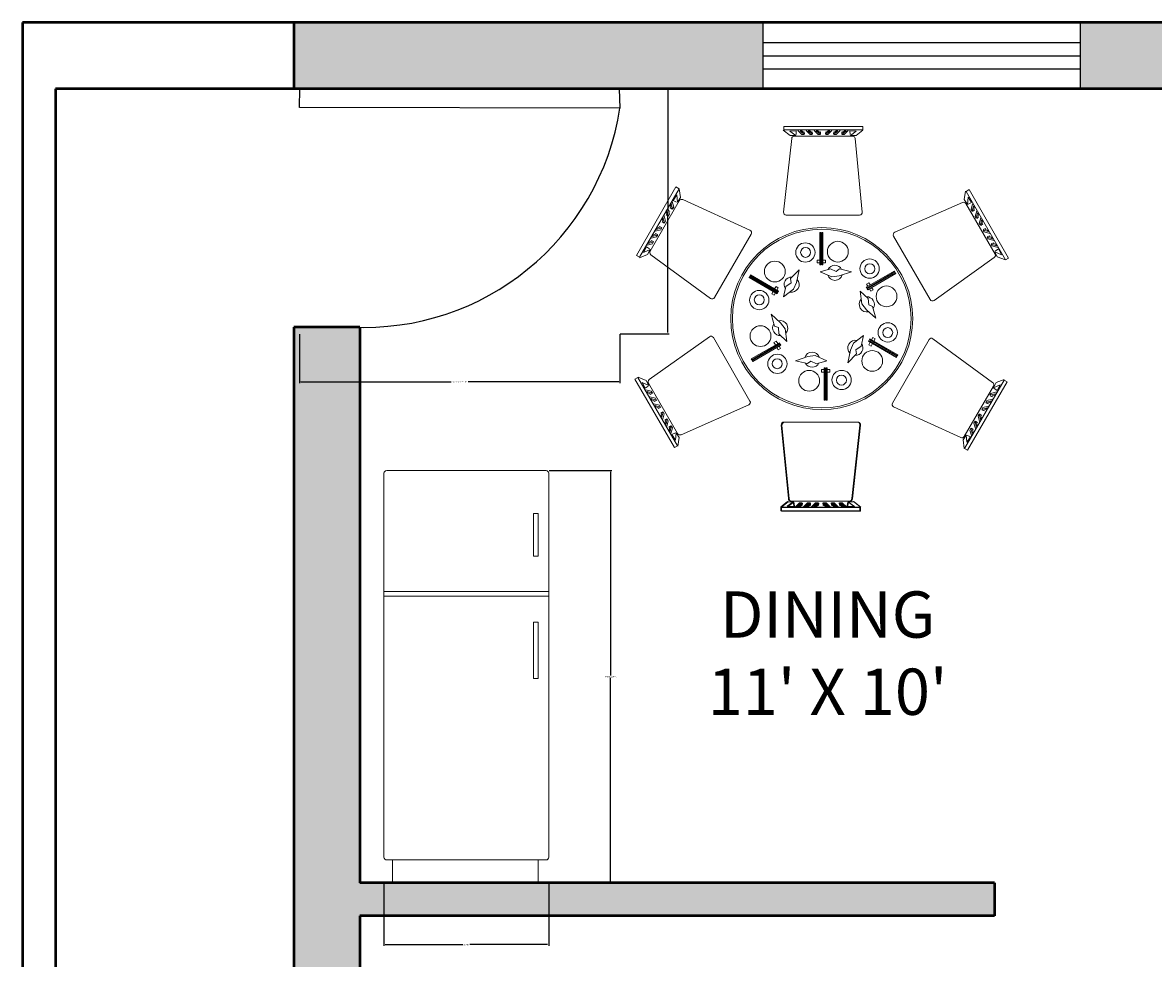
# Model space of a CAD drawing. Units: inches. Extents: x 1771 to 3025, y 319 to 889.
# Tile 19 of 35: x 2219 to 2390, y 747 to 889. Entities that reach past the tile are written whole.
import ezdxf

# ---------------------------------------------------------------- set-up
doc = ezdxf.new("R2010")
doc.units = ezdxf.units.IN
doc.header["$MEASUREMENT"] = 0
for name, color, linetype, lineweight in [('A-ANNO-DIMS', 2, 'Continuous', 18), ('A-AREA-IDEN', 241, 'Continuous', 25), ('A-DOOR', 4, 'Continuous', 25), ('A-FURN', 8, 'Continuous', 18), ('A-GLAZ', 40, 'Continuous', 25), ('A-WALL', 7, 'Continuous', 50), ('A-WALL-PATT', 254, 'Continuous', 13)]:
    doc.layers.add(name, color=color, linetype=linetype, lineweight=lineweight)
doc.styles.get("Standard").update_dxf_attribs({"font": 'arial.ttf'})
doc.dimstyles.get("Standard").update_dxf_attribs({"dimtxt": 0.18, "dimasz": 0.18, "dimexe": 0.18, "dimexo": 0.0625, "dimgap": 0.09, "dimtad": 0, "dimtih": 1, "dimtoh": 1, "dimdec": 4, "dimzin": 0, "dimdsep": 46, "dimtxsty": 'Standard', "dimcen": 0.09, "dimadec": 0, "dimazin": 0, "dimtfac": 1, "dimtdec": 4, "dimtofl": 0, "dimtmove": 0, "dimatfit": 3, "dimfxl": 1, "dimtolj": 1, "dimtzin": 0, "dimarcsym": 0})

# ---------------------------------------------------------------- blocks, each defined once
blk = doc.blocks.new('A$C1C317F9A')
for p, q in [((0.8756, 2.2462), (0.9155, 2.2143)), ((0.8788, 2.2685), (0.8788, 2.2478)), ((1.3449, 2.2685), (0.8788, 2.2685)), ((0.8788, 2.2478), (1.3449, 2.2478)), ((0.9139, 2.2414), (0.9522, 2.243)), ((0.949, 2.2159), (0.9139, 2.2414)), ((0.9155, 2.2143), (0.949, 2.2159)), ((0.941, 2.2111), (1.2841, 2.2111)), ((0.9522, 2.243), (0.9506, 2.2206)), ((0.9618, 2.2446), (0.9857, 2.2206)), ((0.9745, 2.243), (0.9841, 2.243)), ((0.9985, 2.2206), (0.9745, 2.243)), ((0.9841, 2.243), (0.9953, 2.2334)), ((0.9857, 2.2206), (0.9985, 2.2206)), ((0.9953, 2.2334), (0.9985, 2.2366)), ((0.9985, 2.2366), (1.0001, 2.2222)), ((1.0097, 2.2446), (1.0336, 2.2206)), ((1.0224, 2.243), (1.032, 2.243)), ((1.0464, 2.2206), (1.0224, 2.243)), ((1.032, 2.243), (1.0432, 2.2334)), ((1.0336, 2.2206), (1.0464, 2.2206)), ((1.0432, 2.2334), (1.0464, 2.2366)), ((1.0464, 2.2366), (1.048, 2.2222)), ((1.0576, 2.2446), (1.0815, 2.2206)), ((1.0703, 2.243), (1.0799, 2.243)), ((1.0943, 2.2206), (1.0703, 2.243)), ((1.0799, 2.243), (1.0911, 2.2334)), ((1.0815, 2.2206), (1.0943, 2.2206)), ((1.0911, 2.2334), (1.0943, 2.2366)), ((1.0943, 2.2366), (1.0959, 2.2222)), ((1.1262, 2.2366), (1.1246, 2.2222)), ((1.1262, 2.2206), (1.1502, 2.243)), ((1.1294, 2.2334), (1.1262, 2.2366)), ((1.139, 2.2206), (1.1262, 2.2206)), ((1.1406, 2.243), (1.1294, 2.2334)), ((1.1629, 2.2446), (1.139, 2.2206)), ((1.1502, 2.243), (1.1406, 2.243)), ((1.1741, 2.2366), (1.1725, 2.2222)), ((1.1741, 2.2206), (1.1981, 2.243)), ((1.1773, 2.2334), (1.1741, 2.2366)), ((1.1869, 2.2206), (1.1741, 2.2206)), ((1.1885, 2.243), (1.1773, 2.2334)), ((1.2108, 2.2446), (1.1869, 2.2206)), ((1.1981, 2.243), (1.1885, 2.243)), ((1.222, 2.2366), (1.2204, 2.2222)), ((1.222, 2.2206), (1.246, 2.243)), ((1.2252, 2.2334), (1.222, 2.2366)), ((1.2348, 2.2206), (1.222, 2.2206)), ((1.2364, 2.243), (1.2252, 2.2334)), ((1.2587, 2.2446), (1.2348, 2.2206)), ((1.246, 2.243), (1.2364, 2.243)), ((1.2683, 2.243), (1.2699, 2.2206)), ((1.3066, 2.2414), (1.2683, 2.243)), ((1.2715, 2.2159), (1.3066, 2.2414)), ((1.305, 2.2143), (1.2715, 2.2159)), ((1.3449, 2.2462), (1.305, 2.2143)), ((1.3449, 2.2478), (1.3449, 2.2685)), ((0.8775, 1.7628), (0.9251, 2.1968)), ((1.3, 2.1966), (1.3417, 1.7626)), ((0.2422, 1.9115), (0.0091, 1.5078)), ((0.0271, 1.4974), (0.2602, 1.9011)), ((0.2602, 1.9011), (0.2422, 1.9115)), ((0.2615, 1.9003), (0.2692, 1.8498)), ((1.9514, 1.8873), (1.9438, 1.8368)), ((1.9724, 1.8957), (1.9544, 1.8854)), ((1.9544, 1.8854), (2.1875, 1.4816)), ((2.2055, 1.492), (1.9724, 1.8957)), ((0.09, 1.5329), (0.2615, 1.8301)), ((0.2148, 1.813), (0.21, 1.8047)), ((0.21, 1.8047), (0.2127, 1.7903)), ((0.2222, 1.7811), (0.2148, 1.813)), ((0.2198, 1.8249), (0.2286, 1.7922)), ((0.2465, 1.8648), (0.226, 1.8324)), ((0.226, 1.8324), (0.2461, 1.8226)), ((0.2511, 1.8216), (0.2465, 1.8648)), ((0.2692, 1.8498), (0.2511, 1.8216)), ((0.282, 1.8367), (0.6787, 1.6557)), ((1.5338, 1.644), (1.9335, 1.8198)), ((1.9438, 1.8368), (1.9619, 1.8086)), ((1.9537, 1.8131), (2.1253, 1.516)), ((1.9619, 1.8086), (1.9665, 1.8518)), ((1.9665, 1.8518), (1.987, 1.8194)), ((1.987, 1.8194), (1.9669, 1.8096)), ((1.9932, 1.8119), (1.9844, 1.7792)), ((0.1719, 1.7419), (0.1807, 1.7092)), ((0.1888, 1.7488), (0.1844, 1.7476)), ((0.1844, 1.7476), (0.1961, 1.7391)), ((0.1909, 1.7716), (0.1861, 1.7633)), ((0.1861, 1.7633), (0.1888, 1.7488)), ((0.1982, 1.7396), (0.1909, 1.7716)), ((0.1959, 1.7834), (0.2046, 1.7507)), ((0.2046, 1.7507), (0.1982, 1.7396)), ((0.2127, 1.7903), (0.2084, 1.7891)), ((0.2084, 1.7891), (0.22, 1.7805)), ((0.2286, 1.7922), (0.2222, 1.7811)), ((1.3258, 1.7451), (0.8934, 1.7451)), ((1.9844, 1.7792), (1.9908, 1.7681)), ((1.9908, 1.7681), (1.9982, 1.8)), ((2.0046, 1.7761), (1.993, 1.7675)), ((1.9982, 1.8), (2.003, 1.7917)), ((2.003, 1.7917), (2.0003, 1.7773)), ((2.0003, 1.7773), (2.0046, 1.7761)), ((2.0171, 1.7704), (2.0084, 1.7377)), ((2.0084, 1.7377), (2.0147, 1.7266)), ((2.0147, 1.7266), (2.0221, 1.7585)), ((2.0221, 1.7585), (2.0269, 1.7502)), ((2.0269, 1.7502), (2.0242, 1.7358)), ((2.0242, 1.7358), (2.0286, 1.7346)), ((0.1583, 1.6705), (0.127, 1.6609)), ((0.127, 1.6609), (0.1318, 1.6692)), ((0.1318, 1.6692), (0.1457, 1.6741)), ((0.1445, 1.6785), (0.1577, 1.6727)), ((0.1457, 1.6741), (0.1445, 1.6785)), ((0.1519, 1.6595), (0.1583, 1.6705)), ((0.1648, 1.7073), (0.1605, 1.7061)), ((0.1605, 1.7061), (0.1721, 1.6976)), ((0.1669, 1.7301), (0.1621, 1.7218)), ((0.1621, 1.7218), (0.1648, 1.7073)), ((0.1743, 1.6982), (0.1669, 1.7301)), ((0.1807, 1.7092), (0.1743, 1.6982)), ((2.0286, 1.7346), (2.0169, 1.726)), ((2.0411, 1.7289), (2.0323, 1.6962)), ((2.0323, 1.6962), (2.0387, 1.6852)), ((2.0387, 1.6852), (2.0461, 1.7171)), ((2.0525, 1.6931), (2.0409, 1.6846)), ((2.0461, 1.7171), (2.0509, 1.7088)), ((2.0509, 1.7088), (2.0482, 1.6943)), ((2.0482, 1.6943), (2.0525, 1.6931)), ((0.0953, 1.6092), (0.128, 1.618)), ((0.1344, 1.629), (0.1031, 1.6195)), ((0.1031, 1.6195), (0.1078, 1.6278)), ((0.1078, 1.6278), (0.1217, 1.6327)), ((0.1192, 1.6507), (0.1519, 1.6595)), ((0.1217, 1.6327), (0.1206, 1.637)), ((0.1206, 1.637), (0.1338, 1.6312)), ((0.128, 1.618), (0.1344, 1.629)), ((0.6859, 1.6332), (0.4697, 1.2588)), ((1.091, 1.6437, 0.0908), (1.091, 1.4528, 0.0908)), ((1.097, 1.6437, 0.0908), (1.091, 1.6437, 0.0908)), ((1.097, 1.4528, 0.0908), (1.097, 1.6437, 0.0908)), ((1.1023, 1.6437, 0.0908), (1.1023, 1.4528, 0.0908)), ((1.1083, 1.6437, 0.0908), (1.1023, 1.6437, 0.0908)), ((1.1083, 1.4528, 0.0908), (1.1083, 1.6437, 0.0908)), ((1.7426, 1.2469), (1.5264, 1.6214)), ((2.0547, 1.6575), (2.086, 1.6479)), ((2.061, 1.6464), (2.0547, 1.6575)), ((2.0685, 1.6655), (2.0552, 1.6597)), ((2.0937, 1.6377), (2.061, 1.6464)), ((2.0673, 1.6611), (2.0685, 1.6655)), ((2.0812, 1.6562), (2.0673, 1.6611)), ((2.0786, 1.616), (2.1099, 1.6065)), ((2.085, 1.605), (2.0786, 1.616)), ((2.0924, 1.624), (2.0792, 1.6182)), ((2.086, 1.6479), (2.0812, 1.6562)), ((2.1177, 1.5962), (2.085, 1.605)), ((2.0913, 1.6196), (2.0924, 1.624)), ((2.1051, 1.6148), (2.0913, 1.6196)), ((2.1099, 1.6065), (2.1051, 1.6148)), ((0.0502, 1.5246), (0.0679, 1.5586)), ((0.0898, 1.5423), (0.0502, 1.5246)), ((0.0679, 1.5586), (0.0865, 1.5461)), ((0.0713, 1.5677), (0.104, 1.5765)), ((0.0745, 1.5125), (0.0898, 1.5423)), ((0.1104, 1.5876), (0.0791, 1.578)), ((0.0791, 1.578), (0.0839, 1.5863)), ((0.0839, 1.5863), (0.0978, 1.5912)), ((0.0966, 1.5955), (0.1098, 1.5897)), ((0.0978, 1.5912), (0.0966, 1.5955)), ((0.104, 1.5765), (0.1104, 1.5876)), ((2.1026, 1.5745), (2.1339, 1.565)), ((2.1089, 1.5635), (2.1026, 1.5745)), ((2.1164, 1.5825), (2.1031, 1.5767)), ((2.1416, 1.5547), (2.1089, 1.5635)), ((2.1152, 1.5782), (2.1164, 1.5825)), ((2.1291, 1.5733), (2.1152, 1.5782)), ((2.145, 1.5456), (2.1265, 1.5331)), ((2.1339, 1.565), (2.1291, 1.5733)), ((2.1628, 1.5116), (2.145, 1.5456)), ((0.0091, 1.5078), (0.0271, 1.4974)), ((0.0269, 1.4939), (0.0745, 1.5125)), ((0.4464, 1.2539), (0.0943, 1.5121)), ((1.0755, 1.4796, 0.0908), (1.0755, 1.4641, 0.0908)), ((1.091, 1.4796, 0.0908), (1.0755, 1.4796, 0.0908)), ((1.1023, 1.4796, 0.0908), (1.097, 1.4796, 0.0908)), ((1.125, 1.4796, 0.0908), (1.1083, 1.4796, 0.0908)), ((1.125, 1.4641, 0.0908), (1.125, 1.4796, 0.0908)), ((2.1208, 1.495), (1.7657, 1.2419)), ((2.1232, 1.5293), (2.1628, 1.5116)), ((2.1385, 1.4995), (2.1232, 1.5293)), ((2.1861, 1.4809), (2.1385, 1.4995)), ((2.1875, 1.4816), (2.2055, 1.492)), ((0.9684, 1.4231, 0.0908), (0.9184, 1.3706, 0.0908)), ((0.953, 1.3489, 0.0908), (0.9684, 1.4231, 0.0908)), ((1.0755, 1.4641, 0.0908), (1.091, 1.4641, 0.0908)), ((1.091, 1.4528, 0.0908), (1.097, 1.4528, 0.0908)), ((1.1549, 1.429, 0.0908), (1.0933, 1.4112, 0.0908)), ((1.0933, 1.4112, 0.0908), (1.1623, 1.3815, 0.0908)), ((1.097, 1.4641, 0.0908), (1.1023, 1.4641, 0.0908)), ((1.1023, 1.4528, 0.0908), (1.1083, 1.4528, 0.0908)), ((1.1083, 1.4641, 0.0908), (1.125, 1.4641, 0.0908)), ((1.1882, 1.4134, 0.0908), (1.1549, 1.429, 0.0908)), ((1.2075, 1.4282, 0.0908), (1.1882, 1.4134, 0.0908)), ((1.2061, 1.3874, 0.0908), (1.278, 1.4112, 0.0908)), ((1.278, 1.4112, 0.0908), (1.2075, 1.4282, 0.0908)), ((1.5304, 1.4154, 0.0908), (1.365, 1.3199, 0.0908)), ((1.368, 1.3147, 0.0908), (1.5334, 1.4102, 0.0908)), ((1.5361, 1.4055, 0.0908), (1.3707, 1.3101, 0.0908)), ((1.5334, 1.4102, 0.0908), (1.5304, 1.4154, 0.0908)), ((1.539, 1.4004, 0.0908), (1.5361, 1.4055, 0.0908)), ((0.6765, 1.3825, 0.0908), (0.6735, 1.3774, 0.0908)), ((0.6735, 1.3774, 0.0908), (0.8389, 1.2819, 0.0908)), ((0.8419, 1.2871, 0.0908), (0.6765, 1.3825, 0.0908)), ((0.6822, 1.3924, 0.0908), (0.6792, 1.3872, 0.0908)), ((0.6792, 1.3872, 0.0908), (0.8446, 1.2917, 0.0908)), ((0.8476, 1.2969, 0.0908), (0.6822, 1.3924, 0.0908)), ((0.9216, 1.3464, 0.0908), (0.8914, 1.3253, 0.0908)), ((0.9184, 1.3706, 0.0908), (0.9216, 1.3464, 0.0908)), ((0.9363, 1.308, 0.0908), (0.953, 1.3489, 0.0908)), ((1.1623, 1.3815, 0.0908), (1.2061, 1.3874, 0.0908)), ((1.3805, 1.3467, 0.0908), (1.3671, 1.339, 0.0908)), ((1.3671, 1.339, 0.0908), (1.3748, 1.3255, 0.0908)), ((1.3737, 1.3049, 0.0908), (1.539, 1.4004, 0.0908)), ((1.3883, 1.3333, 0.0908), (1.3805, 1.3467, 0.0908)), ((0.8156, 1.2953, 0.0908), (0.8079, 1.2819, 0.0908)), ((0.8079, 1.2819, 0.0908), (0.8213, 1.2741, 0.0908)), ((0.8213, 1.3051, 0.0908), (0.8186, 1.3005, 0.0908)), ((0.8213, 1.2741, 0.0908), (0.8291, 1.2876, 0.0908)), ((0.8327, 1.3248, 0.0908), (0.8243, 1.3103, 0.0908)), ((0.8321, 1.2927, 0.0908), (0.8348, 1.2974, 0.0908)), ((0.8461, 1.317, 0.0908), (0.8327, 1.3248, 0.0908)), ((0.8377, 1.3025, 0.0908), (0.8461, 1.317, 0.0908)), ((0.8389, 1.2819, 0.0908), (0.8419, 1.2871, 0.0908)), ((0.8446, 1.2917, 0.0908), (0.8476, 1.2969, 0.0908)), ((0.8914, 1.3253, 0.0908), (0.8761, 1.2631, 0.0908)), ((0.8761, 1.2631, 0.0908), (0.9363, 1.308, 0.0908)), ((1.3763, 1.2527, 0.0908), (1.3301, 1.2971, 0.0908)), ((1.3301, 1.2971, 0.0908), (1.3389, 1.2225, 0.0908)), ((1.365, 1.3199, 0.0908), (1.368, 1.3147, 0.0908)), ((1.3707, 1.3101, 0.0908), (1.3737, 1.3049, 0.0908)), ((1.3778, 1.3204, 0.0908), (1.3805, 1.3157, 0.0908)), ((1.3835, 1.3106, 0.0908), (1.3918, 1.2961, 0.0908)), ((1.3939, 1.3235, 0.0908), (1.3912, 1.3281, 0.0908)), ((1.3918, 1.2961, 0.0908), (1.4053, 1.3038, 0.0908)), ((1.4053, 1.3038, 0.0908), (1.3969, 1.3183, 0.0908)), ((1.3389, 1.2225, 0.0908), (1.366, 1.1876, 0.0908)), ((1.3795, 1.216, 0.0908), (1.3763, 1.2527, 0.0908)), ((1.402, 1.2067, 0.0908), (1.3795, 1.216, 0.0908)), ((1.4225, 1.1371, 0.0908), (1.402, 1.2067, 0.0908)), ((0.8033, 1.1609, 0.0908), (0.8238, 1.0913, 0.0908)), ((0.8599, 1.1105, 0.0908), (0.8033, 1.1609, 0.0908)), ((1.366, 1.1876, 0.0908), (1.4225, 1.1371, 0.0908)), ((0.8238, 1.0913, 0.0908), (0.8463, 1.0821, 0.0908)), ((0.8463, 1.0821, 0.0908), (0.8495, 1.0454, 0.0908)), ((0.8869, 1.0755, 0.0908), (0.8599, 1.1105, 0.0908)), ((0.8957, 1.0009, 0.0908), (0.8869, 1.0755, 0.0908)), ((0.0847, 0.7751), (0.4398, 1.0281)), ((0.4628, 1.0231), (0.679, 0.6486)), ((0.834, 1.0019, 0.0908), (0.8206, 0.9942, 0.0908)), ((0.8424, 0.9875, 0.0908), (0.834, 1.0019, 0.0908)), ((0.8495, 1.0454, 0.0908), (0.8957, 1.0009, 0.0908)), ((1.3498, 1.0349, 0.0908), (1.2896, 0.99, 0.0908)), ((1.3344, 0.9727, 0.0908), (1.3498, 1.0349, 0.0908)), ((1.3813, 1.0063, 0.0908), (1.3783, 1.0011, 0.0908)), ((1.3783, 1.0011, 0.0908), (1.5437, 0.9057, 0.0908)), ((1.5466, 0.9108, 0.0908), (1.3813, 1.0063, 0.0908)), ((1.3869, 1.0161, 0.0908), (1.384, 1.011, 0.0908)), ((1.384, 1.011, 0.0908), (1.5493, 0.9155, 0.0908)), ((1.5523, 0.9207, 0.0908), (1.3869, 1.0161, 0.0908)), ((1.3938, 1.0053, 0.0908), (1.3911, 1.0006, 0.0908)), ((1.4045, 1.0239, 0.0908), (1.3968, 1.0105, 0.0908)), ((1.418, 1.0162, 0.0908), (1.4045, 1.0239, 0.0908)), ((1.4102, 1.0027, 0.0908), (1.418, 1.0162, 0.0908)), ((1.5196, 0.6368), (1.7358, 1.0113)), ((1.7591, 1.0162), (2.1111, 0.7579)), ((0.8522, 0.9931, 0.0908), (0.6868, 0.8977, 0.0908)), ((0.6898, 0.8925, 0.0908), (0.8552, 0.988, 0.0908)), ((0.8578, 0.9833, 0.0908), (0.6925, 0.8878, 0.0908)), ((0.6955, 0.8827, 0.0908), (0.8608, 0.9781, 0.0908)), ((0.8206, 0.9942, 0.0908), (0.8289, 0.9797, 0.0908)), ((0.8319, 0.9745, 0.0908), (0.8346, 0.9699, 0.0908)), ((0.8376, 0.9647, 0.0908), (0.8453, 0.9513, 0.0908)), ((0.848, 0.9776, 0.0908), (0.8453, 0.9823, 0.0908)), ((0.8453, 0.9513, 0.0908), (0.8588, 0.959, 0.0908)), ((0.8588, 0.959, 0.0908), (0.851, 0.9725, 0.0908)), ((0.8552, 0.988, 0.0908), (0.8522, 0.9931, 0.0908)), ((0.8608, 0.9781, 0.0908), (0.8578, 0.9833, 0.0908)), ((1.2728, 0.9491, 0.0908), (1.2574, 0.875, 0.0908)), ((1.2896, 0.99, 0.0908), (1.2728, 0.9491, 0.0908)), ((1.3042, 0.9516, 0.0908), (1.3344, 0.9727, 0.0908)), ((1.3074, 0.9275, 0.0908), (1.3042, 0.9516, 0.0908)), ((1.3881, 0.9955, 0.0908), (1.3797, 0.981, 0.0908)), ((1.3797, 0.981, 0.0908), (1.3932, 0.9732, 0.0908)), ((1.3932, 0.9732, 0.0908), (1.4015, 0.9877, 0.0908)), ((1.4045, 0.9929, 0.0908), (1.4072, 0.9975, 0.0908)), ((0.6868, 0.8977, 0.0908), (0.6898, 0.8925, 0.0908)), ((0.6925, 0.8878, 0.0908), (0.6955, 0.8827, 0.0908)), ((1.0198, 0.9106, 0.0908), (0.9478, 0.8869, 0.0908)), ((0.9478, 0.8869, 0.0908), (1.0183, 0.8698, 0.0908)), ((1.0183, 0.8698, 0.0908), (1.0376, 0.8846, 0.0908)), ((1.0636, 0.9165, 0.0908), (1.0198, 0.9106, 0.0908)), ((1.0376, 0.8846, 0.0908), (1.071, 0.8691, 0.0908)), ((1.1326, 0.8869, 0.0908), (1.0636, 0.9165, 0.0908)), ((1.071, 0.8691, 0.0908), (1.1326, 0.8869, 0.0908)), ((1.2574, 0.875, 0.0908), (1.3074, 0.9275, 0.0908)), ((1.5437, 0.9057, 0.0908), (1.5466, 0.9108, 0.0908)), ((1.5493, 0.9155, 0.0908), (1.5523, 0.9207, 0.0908)), ((1.1175, 0.8339, 0.0908), (1.1008, 0.8339, 0.0908)), ((1.1008, 0.8339, 0.0908), (1.1008, 0.8184, 0.0908)), ((1.1008, 0.8184, 0.0908), (1.1175, 0.8184, 0.0908)), ((1.1235, 0.8453, 0.0908), (1.1175, 0.8453, 0.0908)), ((1.1175, 0.8453, 0.0908), (1.1175, 0.6543, 0.0908)), ((1.1235, 0.6543, 0.0908), (1.1235, 0.8453, 0.0908)), ((1.1289, 0.8339, 0.0908), (1.1235, 0.8339, 0.0908)), ((1.1235, 0.8184, 0.0908), (1.1289, 0.8184, 0.0908)), ((1.1349, 0.8453, 0.0908), (1.1289, 0.8453, 0.0908)), ((1.1289, 0.8453, 0.0908), (1.1289, 0.6543, 0.0908)), ((1.1349, 0.6543, 0.0908), (1.1349, 0.8453, 0.0908)), ((1.1504, 0.8339, 0.0908), (1.1349, 0.8339, 0.0908)), ((1.1349, 0.8184, 0.0908), (1.1504, 0.8184, 0.0908)), ((1.1504, 0.8184, 0.0908), (1.1504, 0.8339, 0.0908)), ((0.018, 0.7884), (0, 0.778)), ((0, 0.778), (0.2331, 0.3743)), ((0.2511, 0.3847), (0.018, 0.7884)), ((0.0193, 0.7892), (0.0669, 0.7706)), ((0.0427, 0.7584), (0.0604, 0.7244)), ((0.0823, 0.7407), (0.0427, 0.7584)), ((0.0604, 0.7244), (0.079, 0.737)), ((0.0669, 0.7706), (0.0823, 0.7407)), ((0.2517, 0.4569), (0.0802, 0.7541)), ((2.1155, 0.7371), (1.9439, 0.4399)), ((2.1784, 0.7726), (1.9453, 0.3689)), ((1.9633, 0.3585), (2.1964, 0.7622)), ((2.131, 0.7576), (2.1156, 0.7277)), ((2.1156, 0.7277), (2.1553, 0.7454)), ((2.1786, 0.7762), (2.131, 0.7576)), ((2.1553, 0.7454), (2.1375, 0.7114)), ((2.1964, 0.7622), (2.1784, 0.7726)), ((0.0638, 0.7153), (0.0965, 0.7066)), ((0.0716, 0.7051), (0.0764, 0.6968)), ((0.1029, 0.6955), (0.0716, 0.7051)), ((0.0764, 0.6968), (0.0903, 0.6919)), ((0.0878, 0.6738), (0.1205, 0.6651)), ((0.0891, 0.6875), (0.1023, 0.6933)), ((0.0903, 0.6919), (0.0891, 0.6875)), ((0.0965, 0.7066), (0.1029, 0.6955)), ((2.1014, 0.6935), (2.095, 0.6825)), ((2.095, 0.6825), (2.1264, 0.6921)), ((2.1089, 0.6745), (2.0956, 0.6803)), ((2.1341, 0.7023), (2.1014, 0.6935)), ((2.1216, 0.6838), (2.1077, 0.6789)), ((2.1077, 0.6789), (2.1089, 0.6745)), ((2.1375, 0.7114), (2.119, 0.724)), ((2.1264, 0.6921), (2.1216, 0.6838)), ((0.0955, 0.6636), (0.1003, 0.6553)), ((0.1269, 0.654), (0.0955, 0.6636)), ((0.1003, 0.6553), (0.1142, 0.6504)), ((0.1117, 0.6324), (0.1444, 0.6236)), ((0.1131, 0.646), (0.1263, 0.6518)), ((0.1142, 0.6504), (0.1131, 0.646)), ((0.1195, 0.6221), (0.1243, 0.6138)), ((0.1508, 0.6125), (0.1195, 0.6221)), ((0.1205, 0.6651), (0.1269, 0.654)), ((0.1243, 0.6138), (0.1382, 0.6089)), ((0.137, 0.6046), (0.1502, 0.6104)), ((0.1382, 0.6089), (0.137, 0.6046)), ((0.1444, 0.6236), (0.1508, 0.6125)), ((0.6716, 0.6261), (0.272, 0.4503)), ((1.1175, 0.6543, 0.0908), (1.1235, 0.6543, 0.0908)), ((1.1289, 0.6543, 0.0908), (1.1349, 0.6543, 0.0908)), ((1.9235, 0.4334), (1.5268, 0.6143)), ((2.0535, 0.6106), (2.0471, 0.5995)), ((2.0471, 0.5995), (2.0785, 0.6091)), ((2.0862, 0.6194), (2.0535, 0.6106)), ((2.0737, 0.6008), (2.0598, 0.5959)), ((2.0775, 0.6521), (2.0711, 0.641)), ((2.0711, 0.641), (2.1024, 0.6506)), ((2.0849, 0.633), (2.0717, 0.6388)), ((2.0785, 0.6091), (2.0737, 0.6008)), ((2.1102, 0.6608), (2.0775, 0.6521)), ((2.0976, 0.6423), (2.0837, 0.6374)), ((2.0837, 0.6374), (2.0849, 0.633)), ((2.1024, 0.6506), (2.0976, 0.6423)), ((0.153, 0.5769), (0.1646, 0.5855)), ((0.1573, 0.5757), (0.153, 0.5769)), ((0.1546, 0.5613), (0.1573, 0.5757)), ((0.1594, 0.553), (0.1546, 0.5613)), ((0.1668, 0.5849), (0.1594, 0.553)), ((0.1644, 0.5411), (0.1732, 0.5738)), ((0.1732, 0.5738), (0.1668, 0.5849)), ((0.1769, 0.5354), (0.1885, 0.544)), ((0.1813, 0.5343), (0.1769, 0.5354)), ((0.1786, 0.5198), (0.1813, 0.5343)), ((0.1907, 0.5434), (0.1834, 0.5115)), ((0.1971, 0.5323), (0.1907, 0.5434)), ((2.0248, 0.5608), (2.0312, 0.5719)), ((2.0336, 0.5281), (2.0248, 0.5608)), ((2.0312, 0.5719), (2.0386, 0.54)), ((2.045, 0.5639), (2.0334, 0.5725)), ((2.0386, 0.54), (2.0433, 0.5483)), ((2.0406, 0.5627), (2.045, 0.5639)), ((2.0433, 0.5483), (2.0406, 0.5627)), ((2.061, 0.5915), (2.0477, 0.5973)), ((2.0598, 0.5959), (2.061, 0.5915)), ((0.1834, 0.5115), (0.1786, 0.5198)), ((0.1884, 0.4996), (0.1971, 0.5323)), ((0.2009, 0.4939), (0.2125, 0.5025)), ((0.2052, 0.4928), (0.2009, 0.4939)), ((0.2025, 0.4783), (0.2052, 0.4928)), ((0.2073, 0.47), (0.2025, 0.4783)), ((0.2147, 0.5019), (0.2073, 0.47)), ((0.2123, 0.4582), (0.2211, 0.4909)), ((0.2211, 0.4909), (0.2147, 0.5019)), ((0.9055, 0.0734), (0.8638, 0.5074)), ((0.9096, 0.0719), (0.8679, 0.5059)), ((0.8797, 0.5249), (1.3121, 0.5249)), ((0.8838, 0.5234), (1.3162, 0.5234)), ((1.328, 0.5072), (1.2804, 0.0732)), ((1.3321, 0.5057), (1.2845, 0.0717)), ((1.9769, 0.4779), (1.9833, 0.4889)), ((1.9857, 0.4451), (1.9769, 0.4779)), ((1.9833, 0.4889), (1.9907, 0.457)), ((1.9971, 0.4809), (1.9855, 0.4895)), ((1.9927, 0.4798), (1.9971, 0.4809)), ((1.9955, 0.4653), (1.9927, 0.4798)), ((2.0009, 0.5193), (2.0072, 0.5304)), ((2.0096, 0.4866), (2.0009, 0.5193)), ((2.0072, 0.5304), (2.0146, 0.4985)), ((2.0211, 0.5224), (2.0094, 0.531)), ((2.0146, 0.4985), (2.0194, 0.5068)), ((2.0167, 0.5212), (2.0211, 0.5224)), ((2.0194, 0.5068), (2.0167, 0.5212)), ((0.2185, 0.4507), (0.2386, 0.4604)), ((0.239, 0.4183), (0.2185, 0.4507)), ((0.2436, 0.4615), (0.239, 0.4183)), ((0.2617, 0.4332), (0.2436, 0.4615)), ((0.254, 0.3827), (0.2617, 0.4332)), ((1.9363, 0.4202), (1.9544, 0.4484)), ((1.9439, 0.3697), (1.9363, 0.4202)), ((1.9544, 0.4484), (1.9589, 0.4053)), ((1.9589, 0.4053), (1.9795, 0.4377)), ((1.9795, 0.4377), (1.9593, 0.4474)), ((1.9907, 0.457), (1.9955, 0.4653)), ((0.2331, 0.3743), (0.2511, 0.3847)), ((1.9453, 0.3689), (1.9633, 0.3585)), ((0.8605, 0.0239), (0.9005, 0.0558)), ((0.8605, 0.0223), (0.8605, 0.0015)), ((1.3267, 0.0223), (0.8605, 0.0223)), ((0.8605, 0.0015), (1.3267, 0.0015)), ((0.8647, 0.0223), (0.9046, 0.0543)), ((0.8647, 0.0207), (0.8647, 0)), ((1.3308, 0.0207), (0.8647, 0.0207)), ((0.8647, 0), (1.3308, 0)), ((0.934, 0.0542), (0.8989, 0.0286)), ((0.8989, 0.0286), (0.9372, 0.027)), ((0.9005, 0.0558), (0.934, 0.0542)), ((0.9381, 0.0527), (0.903, 0.0271)), ((0.903, 0.0271), (0.9413, 0.0255)), ((0.9046, 0.0543), (0.9381, 0.0527)), ((1.2645, 0.059), (0.9213, 0.059)), ((1.2686, 0.0574), (0.9255, 0.0574)), ((0.9372, 0.027), (0.9356, 0.0494)), ((0.9413, 0.0255), (0.9397, 0.0479)), ((0.9468, 0.0255), (0.9707, 0.0494)), ((0.9509, 0.0239), (0.9748, 0.0479)), ((0.9835, 0.0494), (0.9595, 0.027)), ((0.9595, 0.027), (0.9691, 0.027)), ((0.9876, 0.0479), (0.9636, 0.0255)), ((0.9636, 0.0255), (0.9732, 0.0255)), ((0.9691, 0.027), (0.9803, 0.0366)), ((0.9707, 0.0494), (0.9835, 0.0494)), ((0.9732, 0.0255), (0.9844, 0.0351)), ((0.9748, 0.0479), (0.9876, 0.0479)), ((0.9803, 0.0366), (0.9835, 0.0334)), ((0.9835, 0.0334), (0.9851, 0.0478)), ((0.9844, 0.0351), (0.9876, 0.0319)), ((0.9876, 0.0319), (0.9892, 0.0463)), ((0.9946, 0.0255), (1.0186, 0.0494)), ((0.9988, 0.0239), (1.0227, 0.0479)), ((1.0314, 0.0494), (1.0074, 0.027)), ((1.0074, 0.027), (1.017, 0.027)), ((1.0355, 0.0479), (1.0115, 0.0255)), ((1.0115, 0.0255), (1.0211, 0.0255)), ((1.017, 0.027), (1.0282, 0.0366)), ((1.0186, 0.0494), (1.0314, 0.0494)), ((1.0211, 0.0255), (1.0323, 0.0351)), ((1.0227, 0.0479), (1.0355, 0.0479)), ((1.0282, 0.0366), (1.0314, 0.0334)), ((1.0314, 0.0334), (1.033, 0.0478)), ((1.0323, 0.0351), (1.0355, 0.0319)), ((1.0355, 0.0319), (1.0371, 0.0463)), ((1.0425, 0.0255), (1.0665, 0.0494)), ((1.0467, 0.0239), (1.0706, 0.0479)), ((1.0793, 0.0494), (1.0553, 0.027)), ((1.0553, 0.027), (1.0649, 0.027)), ((1.0834, 0.0479), (1.0594, 0.0255)), ((1.0594, 0.0255), (1.069, 0.0255)), ((1.0649, 0.027), (1.0761, 0.0366)), ((1.0665, 0.0494), (1.0793, 0.0494)), ((1.069, 0.0255), (1.0802, 0.0351)), ((1.0706, 0.0479), (1.0834, 0.0479)), ((1.0761, 0.0366), (1.0793, 0.0334)), ((1.0793, 0.0334), (1.0809, 0.0478)), ((1.0802, 0.0351), (1.0834, 0.0319)), ((1.0834, 0.0319), (1.085, 0.0463)), ((1.1112, 0.0334), (1.1096, 0.0478)), ((1.1112, 0.0494), (1.1351, 0.027)), ((1.124, 0.0494), (1.1112, 0.0494)), ((1.1144, 0.0366), (1.1112, 0.0334)), ((1.1153, 0.0319), (1.1137, 0.0463)), ((1.1256, 0.027), (1.1144, 0.0366)), ((1.1153, 0.0479), (1.1393, 0.0255)), ((1.1281, 0.0479), (1.1153, 0.0479)), ((1.1185, 0.0351), (1.1153, 0.0319)), ((1.1297, 0.0255), (1.1185, 0.0351)), ((1.1479, 0.0255), (1.124, 0.0494)), ((1.1351, 0.027), (1.1256, 0.027)), ((1.152, 0.0239), (1.1281, 0.0479)), ((1.1393, 0.0255), (1.1297, 0.0255)), ((1.1591, 0.0334), (1.1575, 0.0478)), ((1.1591, 0.0494), (1.183, 0.027)), ((1.1719, 0.0494), (1.1591, 0.0494)), ((1.1623, 0.0366), (1.1591, 0.0334)), ((1.1632, 0.0319), (1.1616, 0.0463)), ((1.1735, 0.027), (1.1623, 0.0366)), ((1.1632, 0.0479), (1.1872, 0.0255)), ((1.176, 0.0479), (1.1632, 0.0479)), ((1.1664, 0.0351), (1.1632, 0.0319)), ((1.1776, 0.0255), (1.1664, 0.0351)), ((1.1958, 0.0255), (1.1719, 0.0494)), ((1.183, 0.027), (1.1735, 0.027)), ((1.1999, 0.0239), (1.176, 0.0479)), ((1.1872, 0.0255), (1.1776, 0.0255)), ((1.207, 0.0334), (1.2054, 0.0478)), ((1.207, 0.0494), (1.2309, 0.027)), ((1.2198, 0.0494), (1.207, 0.0494)), ((1.2102, 0.0366), (1.207, 0.0334)), ((1.2111, 0.0319), (1.2095, 0.0463)), ((1.2214, 0.027), (1.2102, 0.0366)), ((1.2111, 0.0479), (1.235, 0.0255)), ((1.2239, 0.0479), (1.2111, 0.0479)), ((1.2143, 0.0351), (1.2111, 0.0319)), ((1.2255, 0.0255), (1.2143, 0.0351)), ((1.2437, 0.0255), (1.2198, 0.0494)), ((1.2309, 0.027), (1.2214, 0.027)), ((1.2478, 0.0239), (1.2239, 0.0479)), ((1.235, 0.0255), (1.2255, 0.0255)), ((1.2533, 0.027), (1.2549, 0.0494)), ((1.2916, 0.0286), (1.2533, 0.027)), ((1.29, 0.0558), (1.2565, 0.0542)), ((1.2565, 0.0542), (1.2916, 0.0286)), ((1.2574, 0.0255), (1.259, 0.0479)), ((1.2957, 0.0271), (1.2574, 0.0255)), ((1.2941, 0.0543), (1.2606, 0.0527)), ((1.2606, 0.0527), (1.2957, 0.0271)), ((1.3299, 0.0239), (1.29, 0.0558)), ((1.334, 0.0223), (1.2941, 0.0543)), ((1.3267, 0.0015), (1.3267, 0.0223)), ((1.3308, 0), (1.3308, 0.0207))]:
    blk.add_line(p, q)
for centre, radius in [((1.1027, 1.135), 0.537), ((1.1027, 1.135), 0.527), ((1.0059, 1.525, 0.0908), 0.0569), ((1.0072, 1.5257, 0.0908), 0.0294), ((1.1975, 1.5297, 0.0908), 0.0613), ((0.8256, 1.4126, 0.0908), 0.0613), ((1.385, 1.4297, 0.0908), 0.0569), ((1.3863, 1.4289, 0.0908), 0.0294), ((0.7338, 1.2443, 0.0908), 0.0569), ((0.7339, 1.2458, 0.0908), 0.0294), ((1.4849, 1.2661, 0.0908), 0.0613), ((0.741, 1.0319, 0.0908), 0.0613), ((1.4921, 1.0537, 0.0908), 0.0569), ((1.492, 1.0522, 0.0908), 0.0294), ((1.4003, 0.8854, 0.0908), 0.0613), ((0.8408, 0.8683, 0.0908), 0.0569), ((0.8396, 0.8691, 0.0908), 0.0294), ((1.0283, 0.7683, 0.0908), 0.0613), ((1.2199, 0.773, 0.0908), 0.0569), ((1.2186, 0.7723, 0.0908), 0.0294)]:
    blk.add_circle(centre, radius)
for centre, radius, start, end in [((0.941, 2.1951), 0.016, 90, 173.74283), ((1.2841, 2.1951), 0.016, 5.48012, 90), ((0.2754, 1.8222), 0.016, 65.48012, 150), ((1.9399, 1.8052), 0.016, 30, 113.74283), ((0.8934, 1.7611), 0.016, 173.74283, 270), ((1.3258, 1.7611), 0.016, 270, 5.48012), ((0.6721, 1.6412), 0.016, 330, 65.48012), ((1.5403, 1.6294), 0.016, 113.74283, 210), ((0.1038, 1.525), 0.016, 150, 233.74283), ((2.1115, 1.508), 0.016, 305.48012, 30), ((1.1801, 1.4052, 0.0908), 0.0446, 26.66413, 154.14416), ((0.9246, 1.3353, 0.0908), 0.0446, 86.66413, 214.14416), ((0.9246, 1.3353, 0.0908), 0.0446, 257.0611, 44.06617), ((1.1801, 1.4052, 0.0908), 0.0446, 197.0611, 344.06617), ((0.4559, 1.2667), 0.016, 233.74283, 330), ((1.3684, 1.2189, 0.0908), 0.0446, 137.0611, 284.06617), ((1.3684, 1.2189, 0.0908), 0.0446, 326.66413, 94.14416), ((1.7565, 1.2549), 0.016, 210, 305.48012), ((0.8574, 1.0791, 0.0908), 0.0446, 146.66413, 274.14416), ((0.8574, 1.0791, 0.0908), 0.0446, 317.0611, 104.06617), ((0.449, 1.0151), 0.016, 30, 125.48012), ((1.3012, 0.9627, 0.0908), 0.0446, 77.0611, 224.06617), ((1.7496, 1.0033), 0.016, 53.74283, 150), ((1.0457, 0.8928, 0.0908), 0.0446, 17.0611, 164.06617), ((1.3012, 0.9627, 0.0908), 0.0446, 266.66413, 34.14416), ((1.0457, 0.8928, 0.0908), 0.0446, 206.66413, 334.14416), ((0.094, 0.7621), 0.016, 125.48012, 210), ((2.1017, 0.7451), 0.016, 330, 53.74283), ((0.6652, 0.6407), 0.016, 293.74283, 30), ((1.5334, 0.6288), 0.016, 150, 245.48012), ((0.8797, 0.5089), 0.016, 90, 185.48012), ((0.8838, 0.5074), 0.016, 90, 185.48012), ((1.3121, 0.5089), 0.016, 353.74283, 90), ((1.3162, 0.5074), 0.016, 353.74283, 90), ((0.2656, 0.4649), 0.016, 210, 293.74283), ((1.9301, 0.4479), 0.016, 245.48012, 330), ((0.9213, 0.0749), 0.016, 185.48012, 270), ((0.9255, 0.0734), 0.016, 185.48012, 270), ((1.2645, 0.0749), 0.016, 270, 353.74283), ((1.2686, 0.0734), 0.016, 270, 353.74283)]:
    blk.add_arc(centre, radius, start, end)
blk = doc.blocks.new('A$C43BC2F3A')
for p, q in [((0, 1490.5), (0, 93.5)), ((10, 1500), (590, 1500)), ((600, 1490), (600, 93.5)), ((590, 83.5), (10.3, 83.5)), ((22.6, 83.5), (561, 83.5)), ((30.8, 0), (30.8, 83.5)), ((561, 83.5), (561, 0)), ((561, 0), (30.8, 0))]:
    blk.add_line(p, q)
for points in [[(561, 1344.2), (561, 1188.3), (544.3, 1188.3), (544.3, 1344.2)], [(561, 949), (561, 743), (544.3, 743), (544.3, 949)]]:
    blk.add_lwpolyline(points, close=True)
for points in [[(600, 1060.3), (0, 1060.3)], [(600, 1043.6), (0, 1043.6)]]:
    blk.add_lwpolyline(points)
for centre, radius, start, end in [((10, 1490), 10, 90, 180), ((590, 1490), 10, 0, 90), ((10.5, 94), 10.5, 182.8791, 268.8051), ((590, 93.5), 10, 270, 0)]:
    blk.add_arc(centre, radius, start, end)
blk = doc.blocks.new('DOOR-39')
blk.add_lwpolyline([(48.33, 36.05), (48.44, 33.13), (0, 33.22), (0.05, 36.05)], close=True)
blk.add_arc((9.8, 39.1), 39.1, 267.0753, 351.2184)
blk = doc.blocks.new('WIN-48')
for p, q in [((0, 0), (0, 10)), ((48, 0), (48, 10)), ((0, 7), (48, 7)), ((0, 5), (48, 5)), ((0, 3), (48, 3))]:
    blk.add_line(p, q)
blk = doc.blocks.new('*D34')
at = {"layer": 'A-ANNO-DIMS', "color": 0, "lineweight": -2, "transparency": 16777216}
for p, q in [((2261.05, 841.55), (2261.05, 834.16)), ((2309.49, 841.55), (2309.49, 834.16)), ((2261.23, 834.34), (2283.99, 834.34)), ((2309.31, 834.34), (2286.56, 834.34))]:
    blk.add_line(p, q, dxfattribs=at)
at = {"layer": 'A-ANNO-DIMS', "color": 0, "transparency": 16777216}
for points in [[(2261.23, 834.37), (2261.23, 834.31), (2261.05, 834.34)], [(2309.31, 834.37), (2309.31, 834.31), (2309.49, 834.34)]]:
    blk.add_solid(points, dxfattribs=at)
at = {"layer": 'Defpoints', "color": 0, "transparency": 16777216}
for p in [(2261.05, 841.61), (2309.49, 841.61), (2309.49, 834.34)]:
    blk.add_point(p, dxfattribs=at)
at = {"layer": 'A-ANNO-DIMS', "color": 0, "transparency": 16777216, "insert": (2285.27, 834.34), "char_height": 0.18, "attachment_point": 5}
blk.add_mtext('\\A1;MAIN DOOR 48 TYP.', dxfattribs=at)
blk = doc.blocks.new('*D35')
at = {"layer": 'A-ANNO-DIMS', "color": 0, "lineweight": -2, "transparency": 16777216}
for p, q in [((2309.55, 878.63), (2316.94, 878.63)), ((2316.76, 878.45), (2316.76, 860.3)), ((2316.76, 841.79), (2316.76, 859.94)), ((2309.55, 841.61), (2316.94, 841.61))]:
    blk.add_line(p, q, dxfattribs=at)
at = {"layer": 'A-ANNO-DIMS', "color": 0, "transparency": 16777216}
for points in [[(2316.73, 878.45), (2316.79, 878.45), (2316.76, 878.63)], [(2316.73, 841.79), (2316.79, 841.79), (2316.76, 841.61)]]:
    blk.add_solid(points, dxfattribs=at)
at = {"layer": 'Defpoints', "color": 0, "transparency": 16777216}
for p in [(2309.49, 878.63), (2316.76, 878.63), (2309.49, 841.61)]:
    blk.add_point(p, dxfattribs=at)
at = {"layer": 'A-ANNO-DIMS', "color": 0, "transparency": 16777216, "insert": (2316.76, 860.12), "char_height": 0.18, "attachment_point": 5}
blk.add_mtext('\\A1;37 TYP.', dxfattribs=at)
blk = doc.blocks.new('*D50')
at = {"layer": 'A-ANNO-DIMS', "color": 0, "lineweight": -2, "transparency": 16777216}
for p, q in [((2298.8, 820.94), (2308.26, 820.94)), ((2308.08, 820.76), (2308.08, 789.97)), ((2308.08, 758.81), (2308.08, 789.6)), ((2298.8, 758.63), (2308.26, 758.63))]:
    blk.add_line(p, q, dxfattribs=at)
at = {"layer": 'A-ANNO-DIMS', "color": 0, "transparency": 16777216}
for points in [[(2308.05, 820.76), (2308.11, 820.76), (2308.08, 820.94)], [(2308.05, 758.81), (2308.11, 758.81), (2308.08, 758.63)]]:
    blk.add_solid(points, dxfattribs=at)
at = {"layer": 'Defpoints', "color": 0, "transparency": 16777216}
for p in [(2298.73, 820.94), (2308.08, 820.94), (2298.73, 758.63)]:
    blk.add_point(p, dxfattribs=at)
at = {"layer": 'A-ANNO-DIMS', "color": 0, "transparency": 16777216, "insert": (2308.08, 789.79), "char_height": 0.18, "attachment_point": 5}
blk.add_mtext('\\A1;FRIDGE 62 TYP.', dxfattribs=at)
blk = doc.blocks.new('*D51')
at = {"layer": 'A-ANNO-DIMS', "color": 0, "lineweight": -2, "transparency": 16777216}
for p, q in [((2273.81, 758.57), (2273.81, 749.11)), ((2298.73, 758.57), (2298.73, 749.11)), ((2273.99, 749.29), (2285.74, 749.29)), ((2298.55, 749.29), (2286.8, 749.29))]:
    blk.add_line(p, q, dxfattribs=at)
at = {"layer": 'A-ANNO-DIMS', "color": 0, "transparency": 16777216}
for points in [[(2273.99, 749.32), (2273.99, 749.26), (2273.81, 749.29)], [(2298.55, 749.32), (2298.55, 749.26), (2298.73, 749.29)]]:
    blk.add_solid(points, dxfattribs=at)
at = {"layer": 'Defpoints', "color": 0, "transparency": 16777216}
for p in [(2273.81, 758.63), (2298.73, 758.63), (2298.73, 749.29)]:
    blk.add_point(p, dxfattribs=at)
at = {"layer": 'A-ANNO-DIMS', "color": 0, "transparency": 16777216, "insert": (2286.27, 749.29), "char_height": 0.18, "attachment_point": 5}
blk.add_mtext('\\A1;25 TYP.', dxfattribs=at)

msp = doc.modelspace()

# ---------------------------------------------------------------- hatches: boundary and pattern name
at = {"layer": 'A-WALL-PATT'}
h = msp.add_hatch(color=256, dxfattribs=at)
h.dxf.hatch_style = 1
h.paths.add_polyline_path([(2407.16, 878.63), (2429.21, 878.63), (2429.21, 888.63), (2379.16, 888.63), (2379.16, 878.63), (2402.16, 878.63), (2402.16, 830.63), (2407.16, 830.63)])
h.paths.add_polyline_path([(2520.11, 888.63), (2477.21, 888.63), (2477.21, 878.63), (2498.16, 878.63), (2498.16, 794.63), (2402.16, 794.63), (2402.16, 758.63), (2402.16, 664.63), (2407.16, 664.63), (2407.16, 712), (2407.16, 789.63), (2515.16, 789.63), (2515.16, 794.63), (2503.16, 794.63), (2503.16, 878.63), (2520.11, 878.63)])
h.paths.add_polyline_path([(2561.16, 888.63), (2538.11, 888.63), (2538.11, 878.63), (2551.16, 878.63), (2551.16, 789.63), (2551.16, 768.61), (2561.16, 768.61)])
h.paths.add_polyline_path([(2561.16, 720.61), (2551.16, 720.61), (2551.16, 669.63), (2443.16, 669.63), (2443.16, 664.63), (2462.16, 664.63), (2462.16, 652.63), (2467.16, 652.63), (2467.16, 664.63), (2551.16, 664.63), (2551.16, 649.17), (2561.16, 649.17)])
h.paths.add_polyline_path([(2561.16, 631.17), (2551.16, 631.17), (2551.16, 616.63), (2462.16, 616.63), (2443.16, 616.63), (2443.16, 611.63), (2551.16, 611.63), (2551.16, 581.11), (2561.16, 581.11)])
h.paths.add_polyline_path([(2561.16, 533.11), (2551.16, 533.11), (2551.16, 479.63), (2407.16, 479.63), (2407.16, 616.63), (2397.16, 616.63), (2397.16, 543.63), (2306.16, 543.63), (2306.16, 533.63), (2397.16, 533.63), (2397.16, 469.63), (2551.16, 469.63), (2551.16, 452.76), (2561.16, 452.76)])
h.paths.add_polyline_path([(2561.16, 404.76), (2551.16, 404.76), (2551.16, 393.63), (2397.16, 393.63), (2397.16, 383.63), (2561.16, 383.63)])
h.paths.add_polyline_path([(2270.16, 642.58), (2260.16, 642.58), (2260.16, 533.63), (2270.16, 533.63)])
h.paths.add_polyline_path([(2270.16, 753.63), (2366.16, 753.63), (2366.16, 758.63), (2270.16, 758.63), (2270.16, 842.59, -0.008336), (2268.86, 842.63), (2260.16, 842.63), (2260.16, 690.58), (2270.16, 690.58)])
h.paths.add_polyline_path([(2331.16, 888.63), (2260.16, 888.63), (2260.16, 878.63), (2331.16, 878.63)])

# ---------------------------------------------------------------- linework, layer by layer
at = {"layer": 'A-WALL'}
for p, q in [((2561.16, 888.63), (2219.16, 888.63)), ((2219.16, 888.63), (2219.16, 533.63)), ((2260.16, 888.63), (2260.16, 878.63)), ((2402.16, 878.63), (2224.16, 878.63)), ((2224.16, 878.63), (2224.16, 533.63)), ((2270.16, 842.63), (2260.16, 842.63)), ((2260.16, 842.63), (2260.16, 533.63)), ((2270.16, 842.63), (2270.16, 758.63)), ((2366.16, 758.63), (2270.16, 758.63)), ((2366.16, 758.63), (2366.16, 753.63)), ((2366.16, 753.63), (2270.16, 753.63)), ((2270.16, 753.63), (2270.16, 533.63))]:
    msp.add_line(p, q, dxfattribs=at)

# ---------------------------------------------------------------- block references
at = {"layer": 'A-DOOR'}
msp.add_blockref('DOOR-39', (2261.05, 842.58), dxfattribs=at)
at = {"layer": 'A-FURN'}
for name, p, xscale, yscale, zscale in [('A$C1C317F9A', (2311.76, 814.82), 25.6235517785217, 25.6235517785217, 25.6235517785217), ('A$C43BC2F3A', (2273.81, 758.63), 0.0415387277892195, 0.0415387277892195, 0.0415387277892195)]:
    msp.add_blockref(name, p, dxfattribs=dict(at, xscale=xscale, yscale=yscale, zscale=zscale))
at = {"layer": 'A-GLAZ'}
msp.add_blockref('WIN-48', (2331.16, 878.63), dxfattribs=at)

# ---------------------------------------------------------------- texts
at = {"layer": 'A-AREA-IDEN', "insert": (2298.17, 802.68), "char_height": 7, "attachment_point": 1}
msp.add_mtext_dynamic_manual_height_columns("\\pxqc;DINING \\P11' X 10'", width=85.4611, gutter_width=1, heights=[0], dxfattribs=at)

# ---------------------------------------------------------------- dimensions: what is measured, and where the dimension line sits
at = {"layer": 'A-ANNO-DIMS'}
for base, p1, p2, text, picture, middle in [((2316.76, 878.63), (2309.49, 841.61), (2309.49, 878.63), '<> TYP.', '*D35', (2316.76, 860.12)), ((2308.08, 820.94), (2298.73, 758.63), (2298.73, 820.94), 'FRIDGE <> TYP.', '*D50', (2308.08, 789.79))]:
    dim = msp.add_linear_dim(base=base, p1=p1, p2=p2, angle=90, text=text, dimstyle='Standard', override={"dimdec": 0, "dimrnd": 0, "dimzin": 0, "dimlunit": 2}, dxfattribs=at)
    dim.commit()
    dim.dimension.update_dxf_attribs({"geometry": picture, "text_midpoint": middle})
for base, p1, p2, text, picture, middle in [((2309.49, 834.34), (2261.05, 841.61), (2309.49, 841.61), 'MAIN DOOR <> TYP.', '*D34', (2285.27, 834.34)), ((2298.73, 749.29), (2273.81, 758.63), (2298.73, 758.63), '<> TYP.', '*D51', (2286.27, 749.29))]:
    dim = msp.add_linear_dim(base=base, p1=p1, p2=p2, text=text, dimstyle='Standard', override={"dimdec": 0, "dimrnd": 0, "dimzin": 0, "dimlunit": 2}, dxfattribs=at)
    dim.commit()
    dim.dimension.update_dxf_attribs({"geometry": picture, "text_midpoint": middle})

doc.saveas('drawing.dxf')
